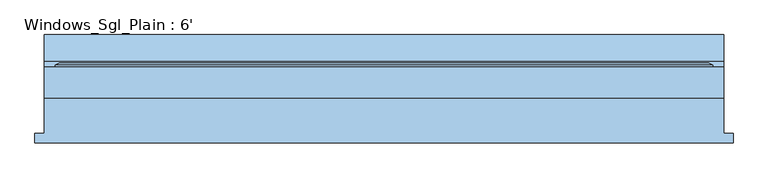
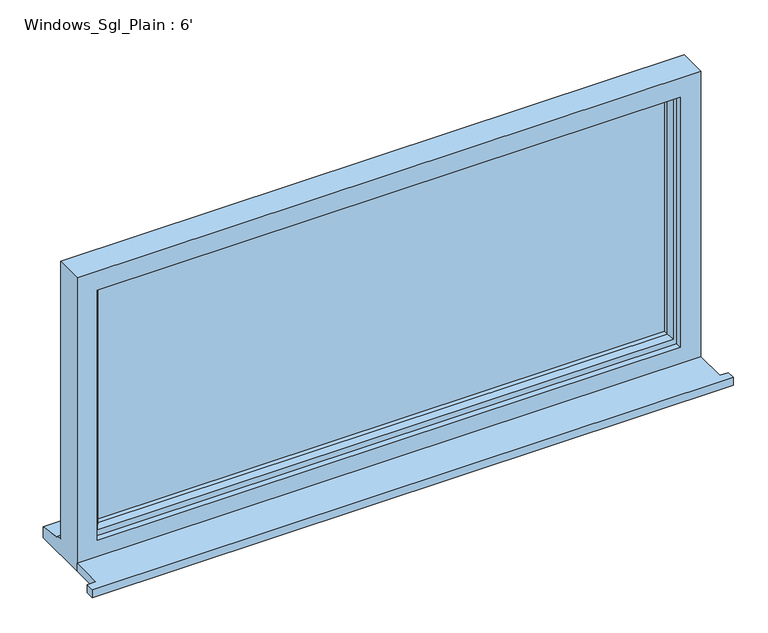
"""IFC4 building model written with IfcOpenShell, lengths in millimetres: window geometry, Windows_Sgl_Plain : 6'."""

from ifc_helpers import new_model, si_unit, frame, origin, place, context, project, spatial, polyline, outline, extrude, faceted_brep, source, transform, mapped, element, save


def windows_sgl_plain_6_060cc830(model_context):
    return source(origin(), model_context, "Body", "SolidModel", [
        extrude(outline(polyline([(-939.4, -130.8434322), (-939.4, -105.8434322), (-914.4, -105.8434322), (-914.4, -10.2434322), (914.4, -10.2434322), (914.4, -105.8434322), (939.4, -105.8434322), (939.4, -130.8434322), (-939.4, -130.8434322)])), frame((0.0, 0.0, 1200.0), z_axis=(0.0, 0.0, 1.0), x_axis=(1.0, 0.0, 0.0)), (0.0, 0.0, 1.0), 25.0),
        faceted_brep([(-914.4, -10.2434322, 1200.0), (914.4, -10.2434322, 1200.0), (914.4, -10.2434322, 2110.0), (-914.4, -10.2434322, 2110.0), (-854.4, -10.2434322, 2050.0), (854.4, -10.2434322, 2050.0), (854.4, -10.2434322, 1275.0), (-854.4, -10.2434322, 1275.0), (-914.4, 72.7565678, 2110.0), (-914.4, 72.7565678, 1251.0), (-914.4, 87.7565678, 1249.68767), (-914.4, 87.7565678, 1244.7449676), (-914.4, 160.2565678, 1233.8088847), (-914.4, 160.2565678, 1200.0), (914.4, 72.7565678, 2110.0), (914.4, 72.7565678, 1251.0), (-874.4, 72.7565678, 2070.0), (-874.4, 72.7565678, 1263.0), (874.4, 72.7565678, 1263.0), (874.4, 72.7565678, 2070.0), (-874.4, 7.7565678, 2070.0), (-874.4, 7.7565678, 1263.0), (874.4, 7.7565678, 2070.0), (874.4, 7.7565678, 1263.0), (-854.4, 7.7565678, 2050.0), (-854.4, 7.7565678, 1275.0), (854.4, 7.7565678, 1275.0), (854.4, 7.7565678, 2050.0), (914.4, 160.2565678, 1200.0), (914.4, 160.2565678, 1233.8088847), (914.4, 87.7565678, 1244.7449676), (914.4, 87.7565678, 1249.68767)], [[[0, 1, 2, 3], [4, 5, 6, 7]], [[0, 3, 8, 9, 10, 11, 12, 13]], [[9, 8, 14, 15], [16, 17, 18, 19]], [[17, 16, 20, 21]], [[20, 22, 23, 21], [24, 25, 26, 27]], [[24, 4, 7, 25]], [[3, 2, 14, 8]], [[16, 19, 22, 20]], [[5, 4, 24, 27]], [[15, 14, 2, 1, 28, 29, 30, 31]], [[19, 18, 23, 22]], [[5, 27, 26, 6]], [[28, 1, 0, 13]], [[29, 28, 13, 12]], [[30, 29, 12, 11]], [[31, 30, 11, 10]], [[15, 31, 10, 9]], [[21, 23, 18, 17]], [[7, 6, 26, 25]]]),
        extrude(outline(polyline([(844.4, 36.7565678), (-844.4, 36.7565678), (-844.4, 60.7565678), (844.4, 60.7565678), (844.4, 36.7565678)])), frame((0.0, 0.0, 1293.0), z_axis=(0.0, 0.0, 1.0), x_axis=(1.0, 0.0, 0.0)), (0.0, 0.0, 1.0), 747.0),
        faceted_brep([(-884.4, 72.7565678, 2080.0), (-884.4, 78.5300705, 2080.0), (-884.4, 78.5300705, 1253.0), (-884.4, 72.7565678, 1253.0), (-874.4, 7.7565678, 2070.0), (-874.4, 72.7565678, 2070.0), (-874.4, 72.7565678, 1263.0), (-874.4, 7.7565678, 1263.0), (-834.4, 22.2494677, 2030.0), (-844.5480377, 7.7565678, 2040.1480377), (-844.5480377, 7.7565678, 1292.8519623), (-834.4, 22.2494677, 1303.0), (-834.4, 36.7565678, 2030.0), (-834.4, 36.7565678, 1303.0), (-844.4, 60.7565678, 2040.0), (-844.4, 36.7565678, 2040.0), (-844.4, 36.7565678, 1293.0), (-844.4, 60.7565678, 1293.0), (-834.4, 78.5300705, 2030.0), (-834.4, 60.7565678, 2030.0), (-834.4, 60.7565678, 1303.0), (-834.4, 78.5300705, 1303.0), (-851.8457548, 84.3035732, 2047.4457548), (-851.8457548, 84.3035732, 1285.5542452), (-873.6153903, 84.3035732, 2069.2153903), (-873.6153903, 84.3035732, 1263.7846097), (884.4, 78.5300705, 1253.0), (884.4, 72.7565678, 1253.0), (874.4, 72.7565678, 1263.0), (874.4, 7.7565678, 1263.0), (844.5480377, 7.7565678, 1292.8519623), (834.4, 22.2494677, 1303.0), (834.4, 36.7565678, 1303.0), (844.4, 36.7565678, 1293.0), (844.4, 60.7565678, 1293.0), (834.4, 60.7565678, 1303.0), (834.4, 78.5300705, 1303.0), (851.8457548, 84.3035732, 1285.5542452), (873.6153903, 84.3035732, 1263.7846097), (884.4, 78.5300705, 2080.0), (884.4, 72.7565678, 2080.0), (874.4, 72.7565678, 2070.0), (874.4, 7.7565678, 2070.0), (844.5480377, 7.7565678, 2040.1480377), (834.4, 22.2494677, 2030.0), (834.4, 36.7565678, 2030.0), (844.4, 36.7565678, 2040.0), (844.4, 60.7565678, 2040.0), (834.4, 60.7565678, 2030.0), (834.4, 78.5300705, 2030.0), (851.8457548, 84.3035732, 2047.4457548), (873.6153903, 84.3035732, 2069.2153903)], [[[0, 1, 2, 3]], [[4, 5, 6, 7]], [[8, 9, 10, 11]], [[12, 8, 11, 13]], [[14, 15, 16, 17]], [[18, 19, 20, 21]], [[22, 18, 21, 23]], [[1, 24, 25, 2]], [[3, 2, 26, 27]], [[7, 6, 28, 29]], [[11, 10, 30, 31]], [[13, 11, 31, 32]], [[17, 16, 33, 34]], [[21, 20, 35, 36]], [[23, 21, 36, 37]], [[2, 25, 38, 26]], [[27, 26, 39, 40]], [[29, 28, 41, 42]], [[31, 30, 43, 44]], [[32, 31, 44, 45]], [[34, 33, 46, 47]], [[36, 35, 48, 49]], [[37, 36, 49, 50]], [[26, 38, 51, 39]], [[40, 39, 1, 0]], [[3, 27, 40, 0], [5, 41, 28, 6]], [[42, 41, 5, 4]], [[7, 29, 42, 4], [9, 43, 30, 10]], [[44, 43, 9, 8]], [[45, 44, 8, 12]], [[15, 46, 33, 16], [13, 32, 45, 12]], [[47, 46, 15, 14]], [[17, 34, 47, 14], [19, 48, 35, 20]], [[49, 48, 19, 18]], [[50, 49, 18, 22]], [[24, 51, 38, 25], [23, 37, 50, 22]], [[39, 51, 24, 1]]]),
    ])


if __name__ == "__main__":
    model = new_model("IFC4")
    model_context = context("Model", 3, world=origin())
    ifc_project = project(units=[si_unit("LENGTHUNIT", "METRE", prefix="MILLI")], contexts=[model_context])
    site = spatial("IfcSite", under=ifc_project)
    building = spatial("IfcBuilding", under=site)
    placement = place(None, origin())
    windows_sgl_plain_6_shape = windows_sgl_plain_6_060cc830(model_context)
    element("IfcWindow", 1, ObjectType="Windows_Sgl_Plain : 6'", at=placement, inside=building, context=model_context, shape_type="MappedRepresentation", body=[
        mapped(windows_sgl_plain_6_shape, transform((0.0, 0.0, 0.0), x_axis=(1.0, 0.0, 0.0), y_axis=(0.0, 1.0, 0.0), z_axis=(0.0, 0.0, 1.0))),
    ])
    save(model, "model.ifc")

# Revit data of these elements
# Type "Windows_Sgl_Plain : 6'"
#   Type Mark = "69"
#   Operation = "SinglePanel"
#   Construction Type Id = "SGL"
#   Manufacturer = "Revit"
#   Keynote = "L10"
#   Analytic Construction = "Large single-glazed windows"
#   Wrap Layers (Ext) from Ext = 0' - 4.03543"
#   Wrap Layers (Int) from Ext = 0' - 6.98819"
#   Window Board Projection = 0' - 0.98425"
#   Window Board Extension = 0' - 0.98425"
#   Visual Light Transmittance = 0.9
#   Solar Heat Gain Coefficient = 0.86
#   Rough Width = 6' - 0"
#   Rough Height = 2' - 11.82677"
#   Height = 2' - 11.82677"
#   Width = 6' - 0"
#   Heat Transfer Coefficient (U) = 5.5617 W/(m²·K)
#   Glazing Thickness = 0' - 0.94488"
#   FrameOffset - External = 0' - 1.9685"
#   Frame Depth = 0' - 2.55906"
#   Default Head Height = 6' - 11.07087"
#   Cill Depth = 0' - 3.44488"
#   Cavity Closer Width = 0' - 1.9685"
#   Cavity Closer Offset from Ext = 0' - 4.03543"
#   Cavity Closer Depth = 0' - 3.34646"
#   Vis - Cavity Closers = yes
#   Define Thermal Properties by = 1
#   Material Trim = Window Frame
#   Material Glass = Glass
#   Material Frame = Window Frame
#   Wall Closure = (empty or 0)
# Element 1 (IfcWindow, "Windows_Sgl_Plain : 6'")
#   Materials on its faces: "Window Frame", "Glass"
# Materials
#   "Window Frame": colour RGB 249 249 249, transparency 0, Keynote = "L10", Cost = 0
#   "Glass": class "Glass", colour RGB 0 128 192, transparency 0.9, Description = "Soda Lime Glass", Cost = 0
